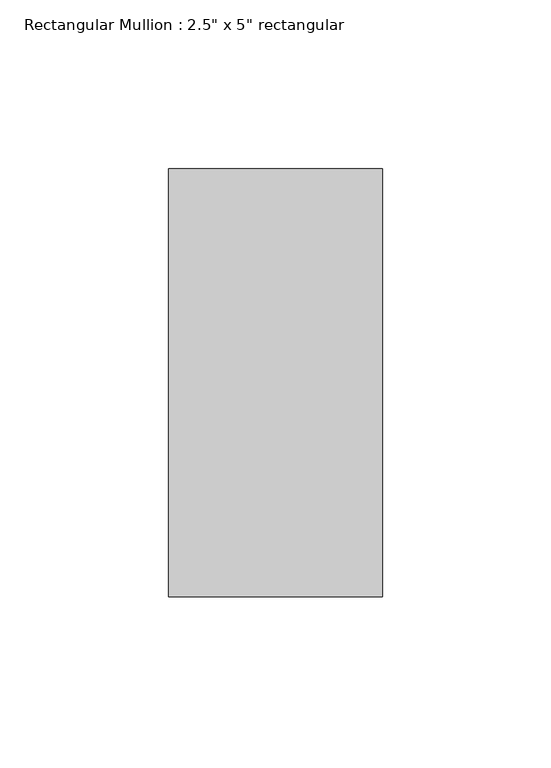
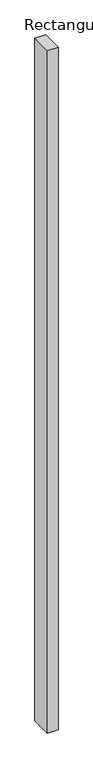
"""IFC4 building model written with IfcOpenShell, lengths in millimetres: member geometry."""

from ifc_helpers import new_model, si_unit, frame, origin, place, context, project, spatial, polyline, outline, extrude, source, transform, mapped, element, save


def member_45b72dba(model_context):
    return source(origin(), model_context, "Body", "SweptSolid", [
        extrude(outline(polyline([(0.0, 63.5), (0.0, -63.5), (-63.5, -63.5), (-63.5, 63.5), (0.0, 63.5)])), frame((0.0, 0.0, -4267.2), z_axis=(0.0, 0.0, 1.0), x_axis=(1.0, 0.0, 0.0)), (0.0, 0.0, 1.0), 4267.2),
    ])


if __name__ == "__main__":
    model = new_model("IFC4")
    model_context = context("Model", 3, world=origin())
    ifc_project = project(units=[si_unit("LENGTHUNIT", "METRE", prefix="MILLI")], contexts=[model_context])
    site = spatial("IfcSite", under=ifc_project)
    building = spatial("IfcBuilding", under=site)
    placement = place(None, origin())
    member_shape = member_45b72dba(model_context)
    element("IfcMember", 1, ObjectType="Rectangular Mullion : 2.5\" x 5\" rectangular", at=placement, inside=building, context=model_context, shape_type="MappedRepresentation", body=[
        mapped(member_shape, transform((0.0, 0.0, 0.0), x_axis=(1.0, 0.0, 0.0), y_axis=(0.0, 1.0, 0.0), z_axis=(0.0, 0.0, 1.0))),
    ])
    save(model, "model.ifc")

# Revit data of these elements
# Type "Rectangular Mullion : 2.5\" x 5\" rectangular"
#   built-in parameter 1007304 = 0.416667 (stored number, unit not read)
#   built-in parameter 1007301 = 0.104167 (stored number, unit not read)
#   built-in parameter 1007300 = 0.104167 (stored number, unit not read)
# Element 1 (IfcMember, "Rectangular Mullion : 2.5\" x 5\" rectangular")
#   Materials on its faces: "Iron, Ductile"
# Materials
#   "Iron, Ductile": class "Metal", colour RGB 0 0 0, transparency 0, Description = "Ductile cast iron", Cost = 0
